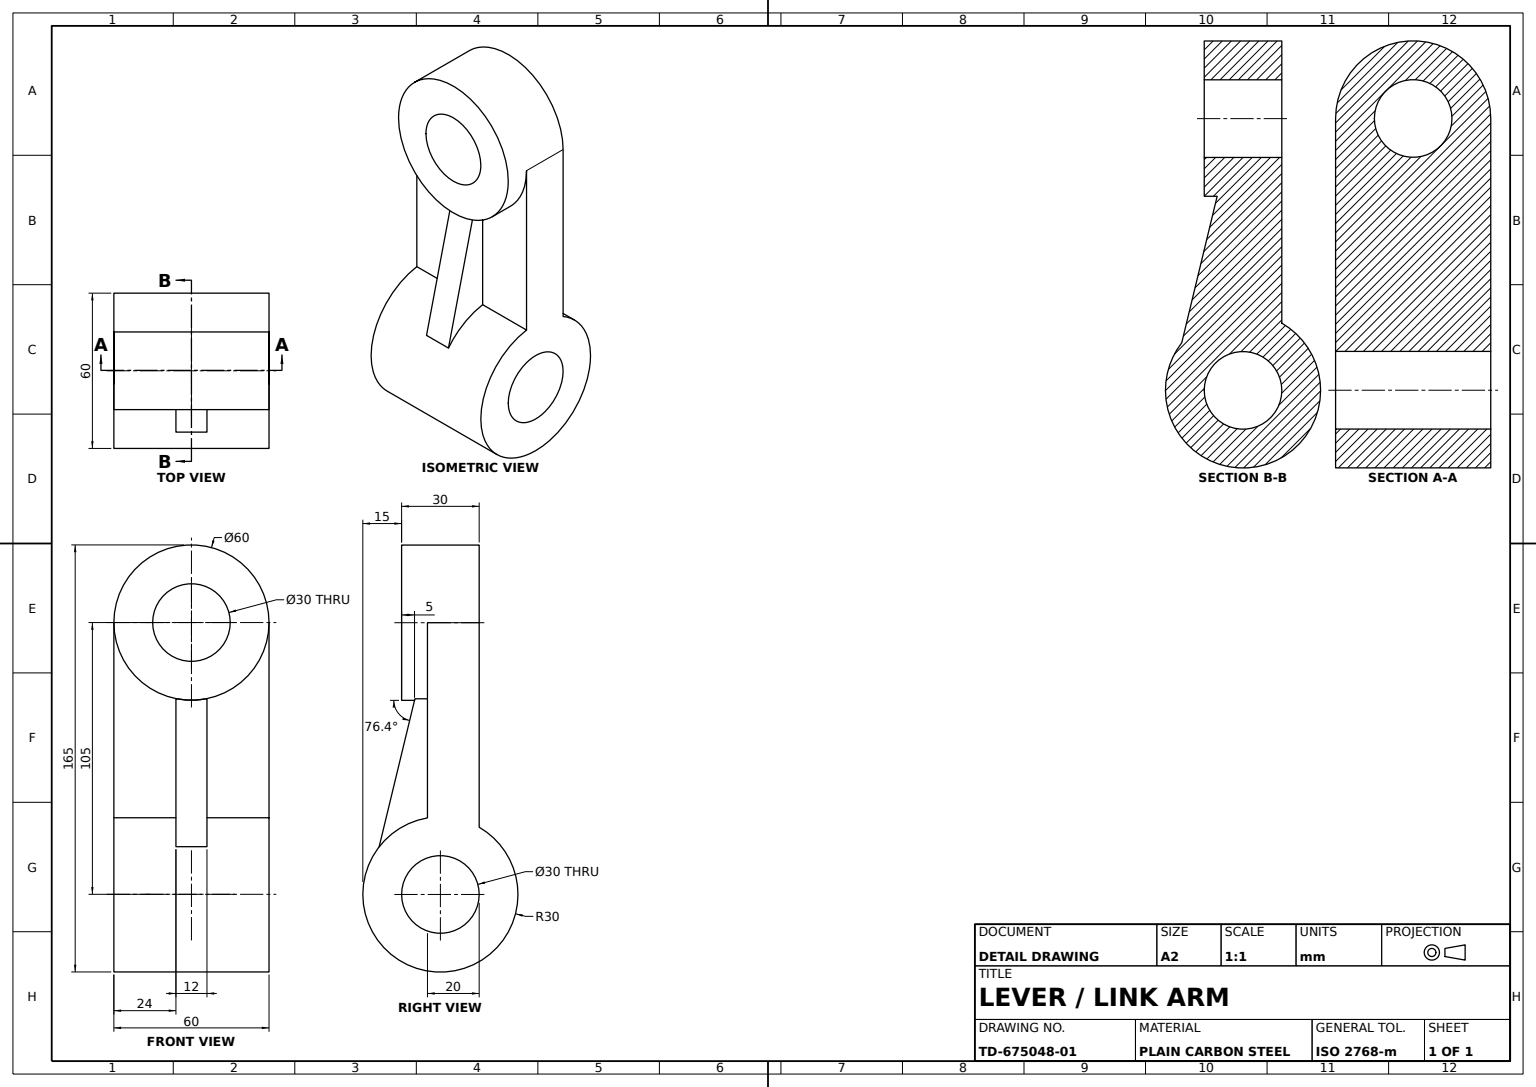
from build123d import *

# Parameters (mm, degrees)
UPPER_EYE_SKETCH_R      = 30
UPPER_EYE_BOSS_DEPTH    = 30
UPPER_EYE_BORE_SKETCH_R = 15
UPPER_EYE_BORE_DEPTH    = 52.961524227
ARM_PROFILE_SKETCH_W    = 20
ARM_PROFILE_SKETCH_H    = 80
ARM_DEPTH               = 30
ARM_START               = 60
ARM_TRIM_CUT_DEPTH      = 60
LOWER_EYE_SKETCH_R      = 30
LOWER_EYE_BOSS_DEPTH    = 30
ARM_RIB_12MM_REACH      = 147.43
ARM_RIB_SKETCH_WALL_W   = 351.093498284
ARM_RIB_SKETCH_WALL_H   = 12
LOWER_EYE_BORE_SKETCH_R = 15
LOWER_EYE_BORE_DEPTH    = 155.434452115


with BuildPart() as part:
    # Upper Eye Sketch → Upper Eye Boss (new body)
    with BuildSketch(Plane.XY):
        Circle(UPPER_EYE_SKETCH_R)
    extrude(amount=UPPER_EYE_BOSS_DEPTH)

    # Upper Eye Bore Sketch → Upper Eye Bore (cut, through all)
    with BuildSketch(Plane.XY.offset(30)):
        Circle(UPPER_EYE_BORE_SKETCH_R)
    extrude(amount=-UPPER_EYE_BORE_DEPTH, mode=Mode.SUBTRACT)

    # Arm Profile Sketch → Arm (add, symmetric)
    with BuildSketch(Plane(origin=(0, 0, 0), x_dir=(0, 0, -1), z_dir=(1, 0, 0))):
        with Locations((-10, -40)):
            Rectangle(ARM_PROFILE_SKETCH_W, ARM_PROFILE_SKETCH_H)
    extrude(amount=ARM_DEPTH, both=True)

    # Arm Trim Sketch → Arm Trim Cut (cut)
    with BuildSketch(Plane.XY.offset(ARM_START)):
        with BuildLine():
            Line((15, 0), (-15, 0))
            ThreePointArc((-15, 0), (0, -15), (15, 0))
        make_face()
    extrude(amount=-ARM_TRIM_CUT_DEPTH, mode=Mode.SUBTRACT)

    # Lower Eye Sketch → Lower Eye Boss (add, symmetric)
    with BuildSketch(Plane(origin=(0, 0, 0), x_dir=(0, 0, -1), z_dir=(1, 0, 0))):
        with Locations((-15, -105)):
            Circle(LOWER_EYE_SKETCH_R)
    extrude(amount=LOWER_EYE_BOSS_DEPTH, both=True)

    # Arm Rib Sketch wall → Arm Rib 12mm (add, up to next)
    with BuildSketch(Plane(origin=(0, -58.299786749, 31.847196974), x_dir=(0, -0.971955050189, 0.235166707705), z_dir=(0, -0.235166707705, -0.971955050189)), mode=Mode.PRIVATE) as arm_rib_12mm_sk1:
        Rectangle(ARM_RIB_SKETCH_WALL_W, ARM_RIB_SKETCH_WALL_H)
    arm_rib_12mm_tool1 = extrude(arm_rib_12mm_sk1.sketch, amount=ARM_RIB_12MM_REACH, mode=Mode.PRIVATE) - part.part
    add(arm_rib_12mm_tool1.solids().sort_by_distance((0, -58.299786749, 31.847196974))[0])

    # Lower Eye Bore Sketch → Lower Eye Bore (cut, through all)
    with BuildSketch(Plane(origin=(30, 0, 0), x_dir=(0, 0, -1), z_dir=(1, 0, 0))):
        with Locations((-15, -105)):
            Circle(LOWER_EYE_BORE_SKETCH_R)
    extrude(amount=-LOWER_EYE_BORE_DEPTH, mode=Mode.SUBTRACT)


solid = part.part
